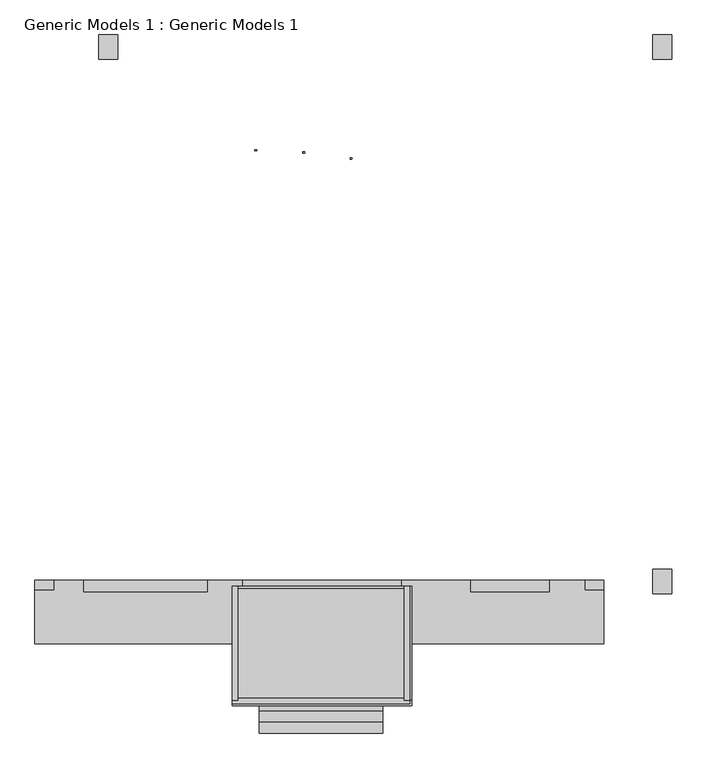
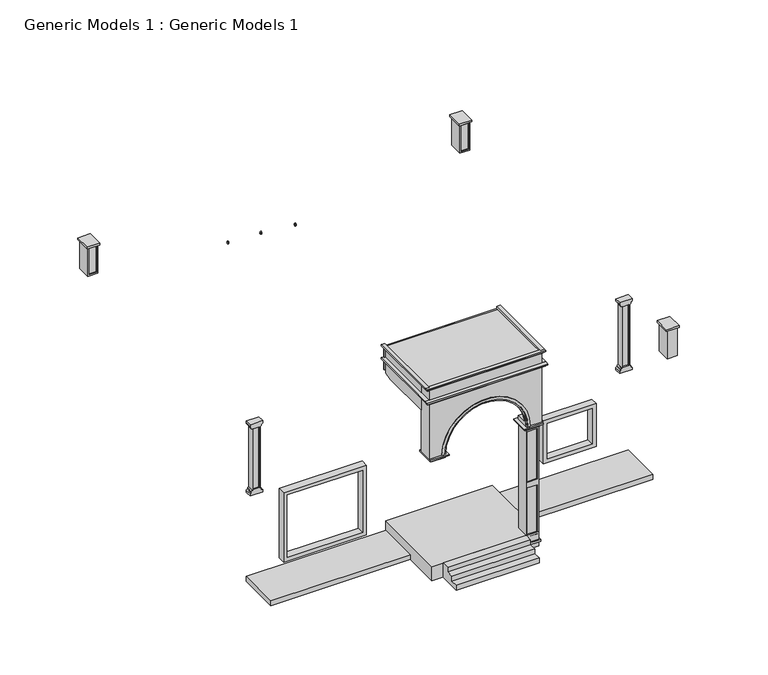
"""IFC4 building model written with IfcOpenShell, lengths in millimetres: proxy geometry, Generic Models 1 : Generic Models 1."""

from ifc_helpers import new_model, si_unit, point, frame, frame_2d, origin, origin_with_axes, place, context, project, spatial, polyline, circle_curve, trimmed, segment, composite_curve, outline, extrude, faceted_brep, source, transform, mapped, element, save
from ifc_brep_helpers import plane_surface, cylinder_surface, revolved_surface, advanced_brep


def generic_models_1_generic_models_1_83f40e1e(model_context):
    return source(origin(), model_context, "Body", "SolidModel", [
        extrude(outline(polyline([(8538.8425759, -5773.6524497), (8538.8425759, -6434.0524497), (8030.8425759, -6434.0524497), (8030.8425759, -5773.6524497), (8538.8425759, -5773.6524497)])), frame((0.0, 0.0, 5029.2), z_axis=(0.0, 0.0, 1.0), x_axis=(1.0, 0.0, 0.0)), (0.0, 0.0, 1.0), 76.2),
        extrude(outline(polyline([(8081.6425759, -6383.2524497), (8081.6425759, -5824.4524497), (8488.0425759, -5824.4524497), (8488.0425759, -6383.2524497), (8081.6425759, -6383.2524497)])), frame((0.0, 0.0, 3810.0), z_axis=(0.0, 0.0, 1.0), x_axis=(1.0, 0.0, 0.0)), (0.0, 0.0, 1.0), 1219.2),
        advanced_brep(
        [(-8670.9249265, -6071.7949916, 6654.8), (-8683.6249265, -6071.7949916, 6654.8), (-8721.7249265, -6071.7949916, 6692.9), (-8721.7249265, -6071.7949916, 6731.0), (-8728.0749265, -6071.7949916, 6731.0), (-8772.5249265, -6071.7949916, 6775.45), (-8772.5249265, -6071.7949916, 6858.0), (-8264.5249265, -6071.7949916, 6858.0), (-8264.5249265, -6071.7949916, 6775.45), (-8308.9749265, -6071.7949916, 6731.0), (-8315.3249265, -6071.7949916, 6731.0), (-8315.3249265, -6071.7949916, 6692.9), (-8353.4249265, -6071.7949916, 6654.8), (-8366.1249265, -6071.7949916, 6654.8), (-8366.1249265, -6071.7949916, 4013.2), (-8353.4249265, -6071.7949916, 4013.2), (-8315.3249265, -6071.7949916, 3975.1), (-8315.3249265, -6071.7949916, 3937.0), (-8308.9749265, -6071.7949916, 3937.0), (-8264.5249265, -6071.7949916, 3892.55), (-8264.5249265, -6071.7949916, 3810.0), (-8772.5249265, -6071.7949916, 3810.0), (-8772.5249265, -6071.7949916, 3892.55), (-8728.0749265, -6071.7949916, 3937.0), (-8721.7249265, -6071.7949916, 3937.0), (-8721.7249265, -6071.7949916, 3975.1), (-8683.6249265, -6071.7949916, 4013.2), (-8670.9249265, -6071.7949916, 4013.2), (-8670.9249265, -6332.4524497, 6654.8), (-8670.9249265, -6332.4524497, 4013.2), (-8683.6249265, -6332.4524497, 4013.2), (-8721.7249265, -6332.4524497, 3975.1), (-8721.7249265, -6332.4524497, 3937.0), (-8728.0749265, -6332.4524497, 3937.0), (-8772.5249265, -6332.4524497, 3892.55), (-8772.5249265, -6332.4524497, 3810.0), (-8264.5249265, -6332.4524497, 3810.0), (-8264.5249265, -6332.4524497, 3892.55), (-8308.9749265, -6332.4524497, 3937.0), (-8315.3249265, -6332.4524497, 3937.0), (-8315.3249265, -6332.4524497, 3975.1), (-8353.4249265, -6332.4524497, 4013.2), (-8366.1249265, -6332.4524497, 4013.2), (-8366.1249265, -6332.4524497, 6654.8), (-8353.4249265, -6332.4524497, 6654.8), (-8315.3249265, -6332.4524497, 6692.9), (-8315.3249265, -6332.4524497, 6731.0), (-8308.9749265, -6332.4524497, 6731.0), (-8264.5249265, -6332.4524497, 6775.45), (-8264.5249265, -6332.4524497, 6858.0), (-8772.5249265, -6332.4524497, 6858.0), (-8772.5249265, -6332.4524497, 6775.45), (-8728.0749265, -6332.4524497, 6731.0), (-8721.7249265, -6332.4524497, 6731.0), (-8721.7249265, -6332.4524497, 6692.9), (-8683.6249265, -6332.4524497, 6654.8), (-8391.5249265, -6332.4524497, 6629.4), (-8391.5249265, -6332.4524497, 4038.6), (-8645.5249265, -6332.4524497, 4038.6), (-8645.5249265, -6332.4524497, 6629.4), (-8391.5249265, -6281.6524497, 6629.4), (-8645.5249265, -6281.6524497, 6629.4), (-8645.5249265, -6281.6524497, 4038.6), (-8391.5249265, -6281.6524497, 4038.6)],
        [
            (0, 1),
            (1, 2, circle_curve(frame((-8683.6249265, -6071.7949916, 6692.9), z_axis=(0.0, 1.0, 0.0), x_axis=(-1.0, 0.0, 0.0)), 38.1)),
            (2, 3),
            (3, 4),
            (4, 5, circle_curve(frame((-8728.0749265, -6071.7949916, 6775.45), z_axis=(0.0, 1.0, 0.0), x_axis=(-1.0, 0.0, 0.0)), 44.45)),
            (5, 6),
            (6, 7),
            (7, 8),
            (8, 9, circle_curve(frame((-8308.9749265, -6071.7949916, 6775.45), z_axis=(0.0, 1.0, 0.0), x_axis=(1.0, 0.0, 0.0)), 44.45)),
            (9, 10),
            (10, 11),
            (11, 12, circle_curve(frame((-8353.4249265, -6071.7949916, 6692.9), z_axis=(0.0, 1.0, 0.0), x_axis=(1.0, 0.0, 0.0)), 38.1)),
            (12, 13),
            (13, 14),
            (14, 15),
            (15, 16, circle_curve(frame((-8353.4249265, -6071.7949916, 3975.1), z_axis=(0.0, 1.0, 0.0), x_axis=(1.0, 0.0, 0.0)), 38.1)),
            (16, 17),
            (17, 18),
            (18, 19, circle_curve(frame((-8308.9749265, -6071.7949916, 3892.55), z_axis=(0.0, 1.0, 0.0), x_axis=(1.0, 0.0, 0.0)), 44.45)),
            (19, 20),
            (20, 21),
            (21, 22),
            (22, 23, circle_curve(frame((-8728.0749265, -6071.7949916, 3892.55), z_axis=(0.0, 1.0, 0.0), x_axis=(-1.0, 0.0, 0.0)), 44.45)),
            (23, 24),
            (24, 25),
            (25, 26, circle_curve(frame((-8683.6249265, -6071.7949916, 3975.1), z_axis=(0.0, 1.0, 0.0), x_axis=(-1.0, 0.0, 0.0)), 38.1)),
            (26, 27),
            (27, 0),
            (28, 29),
            (29, 30),
            (30, 31, circle_curve(frame((-8683.6249265, -6332.4524497, 3975.1), z_axis=(0.0, -1.0, 0.0), x_axis=(-1.0, 0.0, 0.0)), 38.1)),
            (31, 32),
            (32, 33),
            (33, 34, circle_curve(frame((-8728.0749265, -6332.4524497, 3892.55), z_axis=(0.0, -1.0, 0.0), x_axis=(-1.0, 0.0, 0.0)), 44.45)),
            (34, 35),
            (35, 36),
            (36, 37),
            (37, 38, circle_curve(frame((-8308.9749265, -6332.4524497, 3892.55), z_axis=(0.0, -1.0, 0.0), x_axis=(1.0, 0.0, 0.0)), 44.45)),
            (38, 39),
            (39, 40),
            (40, 41, circle_curve(frame((-8353.4249265, -6332.4524497, 3975.1), z_axis=(0.0, -1.0, 0.0), x_axis=(1.0, 0.0, 0.0)), 38.1)),
            (41, 42),
            (42, 43),
            (43, 44),
            (44, 45, circle_curve(frame((-8353.4249265, -6332.4524497, 6692.9), z_axis=(0.0, -1.0, 0.0), x_axis=(1.0, 0.0, 0.0)), 38.1)),
            (45, 46),
            (46, 47),
            (47, 48, circle_curve(frame((-8308.9749265, -6332.4524497, 6775.45), z_axis=(0.0, -1.0, 0.0), x_axis=(1.0, 0.0, 0.0)), 44.45)),
            (48, 49),
            (49, 50),
            (50, 51),
            (51, 52, circle_curve(frame((-8728.0749265, -6332.4524497, 6775.45), z_axis=(0.0, -1.0, 0.0), x_axis=(-1.0, 0.0, 0.0)), 44.45)),
            (52, 53),
            (53, 54),
            (54, 55, circle_curve(frame((-8683.6249265, -6332.4524497, 6692.9), z_axis=(0.0, -1.0, 0.0), x_axis=(-1.0, 0.0, 0.0)), 38.1)),
            (55, 28),
            (56, 57),
            (57, 58),
            (58, 59),
            (59, 56),
            (0, 28),
            (55, 1),
            (54, 2),
            (53, 3),
            (52, 4),
            (51, 5),
            (50, 6),
            (49, 7),
            (48, 8),
            (47, 9),
            (46, 10),
            (45, 11),
            (44, 12),
            (43, 13),
            (42, 14),
            (41, 15),
            (40, 16),
            (39, 17),
            (38, 18),
            (37, 19),
            (36, 20),
            (35, 21),
            (34, 22),
            (33, 23),
            (32, 24),
            (31, 25),
            (30, 26),
            (29, 27),
            (60, 61),
            (61, 62),
            (62, 63),
            (63, 60),
            (63, 57),
            (56, 60),
            (62, 58),
            (61, 59),
        ],
        [
            plane_surface(frame((-8670.9249265, -6071.7949916, 6654.8), z_axis=(0.0, 1.0, 0.0), x_axis=(-1.0, 0.0, 0.0))),
            plane_surface(frame((-8670.9249265, -6332.4524497, 6654.8), z_axis=(0.0, -1.0, 0.0), x_axis=(1.0, 0.0, 0.0))),
            plane_surface(frame((-8670.9249265, -6071.7949916, 6654.8), z_axis=(0.0, 0.0, -1.0), x_axis=(0.0, -1.0, 0.0))),
            cylinder_surface(frame((-8683.6249265, -6332.4524497, 6692.9), z_axis=(0.0, 1.0, 0.0), x_axis=(-1.0, 0.0, 0.0)), 38.1),
            plane_surface(frame((-8721.7249265, -6071.7949916, 6692.9), z_axis=(-1.0, 0.0, 0.0), x_axis=(0.0, -1.0, 0.0))),
            plane_surface(frame((-8721.7249265, -6071.7949916, 6731.0), z_axis=(0.0, 0.0, -1.0), x_axis=(0.0, -1.0, 0.0))),
            cylinder_surface(frame((-8728.0749265, -6332.4524497, 6775.45), z_axis=(0.0, 1.0, 0.0), x_axis=(-1.0, 0.0, 0.0)), 44.45),
            plane_surface(frame((-8772.5249265, -6071.7949916, 6775.45), z_axis=(-1.0, 0.0, 0.0), x_axis=(0.0, -1.0, 0.0))),
            plane_surface(frame((-8772.5249265, -6071.7949916, 6858.0), z_axis=(0.0, 0.0, 1.0), x_axis=(0.0, -1.0, 0.0))),
            plane_surface(frame((-8264.5249265, -6071.7949916, 6858.0), z_axis=(1.0, 0.0, 0.0), x_axis=(0.0, -1.0, 0.0))),
            cylinder_surface(frame((-8308.9749265, -6332.4524497, 6775.45), z_axis=(0.0, 1.0, 0.0), x_axis=(1.0, 0.0, 0.0)), 44.45),
            plane_surface(frame((-8308.9749265, -6071.7949916, 6731.0), z_axis=(0.0, 0.0, -1.0), x_axis=(0.0, -1.0, 0.0))),
            plane_surface(frame((-8315.3249265, -6071.7949916, 6731.0), z_axis=(1.0, 0.0, 0.0), x_axis=(0.0, -1.0, 0.0))),
            cylinder_surface(frame((-8353.4249265, -6332.4524497, 6692.9), z_axis=(0.0, 1.0, 0.0), x_axis=(1.0, 0.0, 0.0)), 38.1),
            plane_surface(frame((-8353.4249265, -6071.7949916, 6654.8), z_axis=(0.0, 0.0, -1.0), x_axis=(0.0, -1.0, 0.0))),
            plane_surface(frame((-8366.1249265, -6071.7949916, 6654.8), z_axis=(1.0, 0.0, 0.0), x_axis=(0.0, -1.0, 0.0))),
            plane_surface(frame((-8366.1249265, -6071.7949916, 4013.2), z_axis=(0.0, 0.0, 1.0), x_axis=(0.0, -1.0, 0.0))),
            cylinder_surface(frame((-8353.4249265, -6332.4524497, 3975.1), z_axis=(0.0, 1.0, 0.0), x_axis=(1.0, 0.0, 0.0)), 38.1),
            plane_surface(frame((-8315.3249265, -6071.7949916, 3975.1), z_axis=(1.0, 0.0, 0.0), x_axis=(0.0, -1.0, 0.0))),
            plane_surface(frame((-8315.3249265, -6071.7949916, 3937.0), z_axis=(0.0, 0.0, 1.0), x_axis=(0.0, -1.0, 0.0))),
            cylinder_surface(frame((-8308.9749265, -6332.4524497, 3892.55), z_axis=(0.0, 1.0, 0.0), x_axis=(1.0, 0.0, 0.0)), 44.45),
            plane_surface(frame((-8264.5249265, -6071.7949916, 3892.55), z_axis=(1.0, 0.0, 0.0), x_axis=(0.0, -1.0, 0.0))),
            plane_surface(frame((-8264.5249265, -6071.7949916, 3810.0), z_axis=(0.0, 0.0, -1.0), x_axis=(0.0, -1.0, 0.0))),
            plane_surface(frame((-8772.5249265, -6071.7949916, 3810.0), z_axis=(-1.0, 0.0, 0.0), x_axis=(0.0, -1.0, 0.0))),
            cylinder_surface(frame((-8728.0749265, -6332.4524497, 3892.55), z_axis=(0.0, 1.0, 0.0), x_axis=(-1.0, 0.0, 0.0)), 44.45),
            plane_surface(frame((-8728.0749265, -6071.7949916, 3937.0), z_axis=(0.0, 0.0, 1.0), x_axis=(0.0, -1.0, 0.0))),
            plane_surface(frame((-8721.7249265, -6071.7949916, 3937.0), z_axis=(-1.0, 0.0, 0.0), x_axis=(0.0, -1.0, 0.0))),
            cylinder_surface(frame((-8683.6249265, -6332.4524497, 3975.1), z_axis=(0.0, 1.0, 0.0), x_axis=(-1.0, 0.0, 0.0)), 38.1),
            plane_surface(frame((-8683.6249265, -6071.7949916, 4013.2), z_axis=(0.0, 0.0, 1.0), x_axis=(0.0, -1.0, 0.0))),
            plane_surface(frame((-8670.9249265, -6071.7949916, 4013.2), z_axis=(-1.0, 0.0, 0.0), x_axis=(0.0, -1.0, 0.0))),
            plane_surface(frame((-8391.5249265, -6281.6524497, 6629.4), z_axis=(0.0, -1.0, 0.0), x_axis=(0.0, 0.0, -1.0))),
            plane_surface(frame((-8391.5249265, -6281.6524497, 6629.4), z_axis=(-1.0, 0.0, 0.0), x_axis=(0.0, -1.0, 0.0))),
            plane_surface(frame((-8391.5249265, -6281.6524497, 4038.6), z_axis=(0.0, 0.0, 1.0), x_axis=(0.0, -1.0, 0.0))),
            plane_surface(frame((-8645.5249265, -6281.6524497, 4038.6), z_axis=(1.0, 0.0, 0.0), x_axis=(0.0, -1.0, 0.0))),
            plane_surface(frame((-8645.5249265, -6281.6524497, 6629.4), z_axis=(0.0, 0.0, -1.0), x_axis=(0.0, -1.0, 0.0))),
        ],
        [
            (0, [[1, 2, 3, 4, 5, 6, 7, 8, 9, 10, 11, 12, 13, 14, 15, 16, 17, 18, 19, 20, 21, 22, 23, 24, 25, 26, 27, 28]]),
            (1, [[29, 30, 31, 32, 33, 34, 35, 36, 37, 38, 39, 40, 41, 42, 43, 44, 45, 46, 47, 48, 49, 50, 51, 52, 53, 54, 55, 56], [57, 58, 59, 60]]),
            (2, [[-1, 61, -56, 62]]),
            (3, [[-2, -62, -55, 63]]),
            (4, [[-3, -63, -54, 64]]),
            (5, [[-4, -64, -53, 65]]),
            (6, [[-5, -65, -52, 66]]),
            (7, [[-6, -66, -51, 67]]),
            (8, [[-7, -67, -50, 68]]),
            (9, [[-8, -68, -49, 69]]),
            (10, [[-9, -69, -48, 70]]),
            (11, [[-10, -70, -47, 71]]),
            (12, [[-11, -71, -46, 72]]),
            (13, [[-12, -72, -45, 73]]),
            (14, [[-13, -73, -44, 74]]),
            (15, [[-14, -74, -43, 75]]),
            (16, [[-15, -75, -42, 76]]),
            (17, [[-16, -76, -41, 77]]),
            (18, [[-17, -77, -40, 78]]),
            (19, [[-18, -78, -39, 79]]),
            (20, [[-19, -79, -38, 80]]),
            (21, [[-20, -80, -37, 81]]),
            (22, [[-21, -81, -36, 82]]),
            (23, [[-22, -82, -35, 83]]),
            (24, [[-23, -83, -34, 84]]),
            (25, [[-24, -84, -33, 85]]),
            (26, [[-25, -85, -32, 86]]),
            (27, [[-26, -86, -31, 87]]),
            (28, [[-27, -87, -30, 88]]),
            (29, [[-28, -88, -29, -61]]),
            (30, [[89, 90, 91, 92]]),
            (31, [[-92, 93, -57, 94]]),
            (32, [[-91, 95, -58, -93]]),
            (33, [[-90, 96, -59, -95]]),
            (34, [[-89, -94, -60, -96]]),
        ],
    ),
        advanced_brep(
        [(6289.6750735, -6071.7949916, 6654.8), (6276.9750735, -6071.7949916, 6654.8), (6238.8750735, -6071.7949916, 6692.9), (6238.8750735, -6071.7949916, 6731.0), (6232.5250735, -6071.7949916, 6731.0), (6188.0750735, -6071.7949916, 6775.45), (6188.0750735, -6071.7949916, 6858.0), (6696.0750735, -6071.7949916, 6858.0), (6696.0750735, -6071.7949916, 6775.45), (6651.6250735, -6071.7949916, 6731.0), (6645.2750735, -6071.7949916, 6731.0), (6645.2750735, -6071.7949916, 6692.9), (6607.1750735, -6071.7949916, 6654.8), (6594.4750735, -6071.7949916, 6654.8), (6594.4750735, -6071.7949916, 4013.2), (6607.1750735, -6071.7949916, 4013.2), (6645.2750735, -6071.7949916, 3975.1), (6645.2750735, -6071.7949916, 3937.0), (6651.6250735, -6071.7949916, 3937.0), (6696.0750735, -6071.7949916, 3892.55), (6696.0750735, -6071.7949916, 3810.0), (6188.0750735, -6071.7949916, 3810.0), (6188.0750735, -6071.7949916, 3892.55), (6232.5250735, -6071.7949916, 3937.0), (6238.8750735, -6071.7949916, 3937.0), (6238.8750735, -6071.7949916, 3975.1), (6276.9750735, -6071.7949916, 4013.2), (6289.6750735, -6071.7949916, 4013.2), (6289.6750735, -6332.4524497, 6654.8), (6289.6750735, -6332.4524497, 4013.2), (6276.9750735, -6332.4524497, 4013.2), (6238.8750735, -6332.4524497, 3975.1), (6238.8750735, -6332.4524497, 3937.0), (6232.5250735, -6332.4524497, 3937.0), (6188.0750735, -6332.4524497, 3892.55), (6188.0750735, -6332.4524497, 3810.0), (6696.0750735, -6332.4524497, 3810.0), (6696.0750735, -6332.4524497, 3892.55), (6651.6250735, -6332.4524497, 3937.0), (6645.2750735, -6332.4524497, 3937.0), (6645.2750735, -6332.4524497, 3975.1), (6607.1750735, -6332.4524497, 4013.2), (6594.4750735, -6332.4524497, 4013.2), (6594.4750735, -6332.4524497, 6654.8), (6607.1750735, -6332.4524497, 6654.8), (6645.2750735, -6332.4524497, 6692.9), (6645.2750735, -6332.4524497, 6731.0), (6651.6250735, -6332.4524497, 6731.0), (6696.0750735, -6332.4524497, 6775.45), (6696.0750735, -6332.4524497, 6858.0), (6188.0750735, -6332.4524497, 6858.0), (6188.0750735, -6332.4524497, 6775.45), (6232.5250735, -6332.4524497, 6731.0), (6238.8750735, -6332.4524497, 6731.0), (6238.8750735, -6332.4524497, 6692.9), (6276.9750735, -6332.4524497, 6654.8), (6569.0750735, -6332.4524497, 6629.4), (6569.0750735, -6332.4524497, 4038.6), (6315.0750735, -6332.4524497, 4038.6), (6315.0750735, -6332.4524497, 6629.4), (6569.0750735, -6281.6524497, 6629.4), (6315.0750735, -6281.6524497, 6629.4), (6315.0750735, -6281.6524497, 4038.6), (6569.0750735, -6281.6524497, 4038.6)],
        [
            (0, 1),
            (1, 2, circle_curve(frame((6276.9750735, -6071.7949916, 6692.9), z_axis=(0.0, 1.0, 0.0), x_axis=(-1.0, 0.0, 0.0)), 38.1)),
            (2, 3),
            (3, 4),
            (4, 5, circle_curve(frame((6232.5250735, -6071.7949916, 6775.45), z_axis=(0.0, 1.0, 0.0), x_axis=(-1.0, 0.0, 0.0)), 44.45)),
            (5, 6),
            (6, 7),
            (7, 8),
            (8, 9, circle_curve(frame((6651.6250735, -6071.7949916, 6775.45), z_axis=(0.0, 1.0, 0.0), x_axis=(1.0, 0.0, 0.0)), 44.45)),
            (9, 10),
            (10, 11),
            (11, 12, circle_curve(frame((6607.1750735, -6071.7949916, 6692.9), z_axis=(0.0, 1.0, 0.0), x_axis=(1.0, 0.0, 0.0)), 38.1)),
            (12, 13),
            (13, 14),
            (14, 15),
            (15, 16, circle_curve(frame((6607.1750735, -6071.7949916, 3975.1), z_axis=(0.0, 1.0, 0.0), x_axis=(1.0, 0.0, 0.0)), 38.1)),
            (16, 17),
            (17, 18),
            (18, 19, circle_curve(frame((6651.6250735, -6071.7949916, 3892.55), z_axis=(0.0, 1.0, 0.0), x_axis=(1.0, 0.0, 0.0)), 44.45)),
            (19, 20),
            (20, 21),
            (21, 22),
            (22, 23, circle_curve(frame((6232.5250735, -6071.7949916, 3892.55), z_axis=(0.0, 1.0, 0.0), x_axis=(-1.0, 0.0, 0.0)), 44.45)),
            (23, 24),
            (24, 25),
            (25, 26, circle_curve(frame((6276.9750735, -6071.7949916, 3975.1), z_axis=(0.0, 1.0, 0.0), x_axis=(-1.0, 0.0, 0.0)), 38.1)),
            (26, 27),
            (27, 0),
            (28, 29),
            (29, 30),
            (30, 31, circle_curve(frame((6276.9750735, -6332.4524497, 3975.1), z_axis=(0.0, -1.0, 0.0), x_axis=(-1.0, 0.0, 0.0)), 38.1)),
            (31, 32),
            (32, 33),
            (33, 34, circle_curve(frame((6232.5250735, -6332.4524497, 3892.55), z_axis=(0.0, -1.0, 0.0), x_axis=(-1.0, 0.0, 0.0)), 44.45)),
            (34, 35),
            (35, 36),
            (36, 37),
            (37, 38, circle_curve(frame((6651.6250735, -6332.4524497, 3892.55), z_axis=(0.0, -1.0, 0.0), x_axis=(1.0, 0.0, 0.0)), 44.45)),
            (38, 39),
            (39, 40),
            (40, 41, circle_curve(frame((6607.1750735, -6332.4524497, 3975.1), z_axis=(0.0, -1.0, 0.0), x_axis=(1.0, 0.0, 0.0)), 38.1)),
            (41, 42),
            (42, 43),
            (43, 44),
            (44, 45, circle_curve(frame((6607.1750735, -6332.4524497, 6692.9), z_axis=(0.0, -1.0, 0.0), x_axis=(1.0, 0.0, 0.0)), 38.1)),
            (45, 46),
            (46, 47),
            (47, 48, circle_curve(frame((6651.6250735, -6332.4524497, 6775.45), z_axis=(0.0, -1.0, 0.0), x_axis=(1.0, 0.0, 0.0)), 44.45)),
            (48, 49),
            (49, 50),
            (50, 51),
            (51, 52, circle_curve(frame((6232.5250735, -6332.4524497, 6775.45), z_axis=(0.0, -1.0, 0.0), x_axis=(-1.0, 0.0, 0.0)), 44.45)),
            (52, 53),
            (53, 54),
            (54, 55, circle_curve(frame((6276.9750735, -6332.4524497, 6692.9), z_axis=(0.0, -1.0, 0.0), x_axis=(-1.0, 0.0, 0.0)), 38.1)),
            (55, 28),
            (56, 57),
            (57, 58),
            (58, 59),
            (59, 56),
            (0, 28),
            (55, 1),
            (54, 2),
            (53, 3),
            (52, 4),
            (51, 5),
            (50, 6),
            (49, 7),
            (48, 8),
            (47, 9),
            (46, 10),
            (45, 11),
            (44, 12),
            (43, 13),
            (42, 14),
            (41, 15),
            (40, 16),
            (39, 17),
            (38, 18),
            (37, 19),
            (36, 20),
            (35, 21),
            (34, 22),
            (33, 23),
            (32, 24),
            (31, 25),
            (30, 26),
            (29, 27),
            (60, 61),
            (61, 62),
            (62, 63),
            (63, 60),
            (63, 57),
            (56, 60),
            (62, 58),
            (61, 59),
        ],
        [
            plane_surface(frame((-8670.9249265, -6071.7949916, 6654.8), z_axis=(0.0, 1.0, 0.0), x_axis=(-1.0, 0.0, 0.0))),
            plane_surface(frame((-8670.9249265, -6332.4524497, 6654.8), z_axis=(0.0, -1.0, 0.0), x_axis=(1.0, 0.0, 0.0))),
            plane_surface(frame((6289.6750735, -6071.7949916, 6654.8), z_axis=(0.0, 0.0, -1.0), x_axis=(0.0, -1.0, 0.0))),
            cylinder_surface(frame((6276.9750735, -5843.1949916, 6692.9), z_axis=(0.0, 1.0, 0.0), x_axis=(-1.0, 0.0, 0.0)), 38.1),
            plane_surface(frame((6238.8750735, -6071.7949916, 6692.9), z_axis=(-1.0, 0.0, 0.0), x_axis=(0.0, -1.0, 0.0))),
            plane_surface(frame((6238.8750735, -6071.7949916, 6731.0), z_axis=(0.0, 0.0, -1.0), x_axis=(0.0, -1.0, 0.0))),
            cylinder_surface(frame((6232.5250735, -5843.1949916, 6775.45), z_axis=(0.0, 1.0, 0.0), x_axis=(-1.0, 0.0, 0.0)), 44.45),
            plane_surface(frame((6188.0750735, -6071.7949916, 6775.45), z_axis=(-1.0, 0.0, 0.0), x_axis=(0.0, -1.0, 0.0))),
            plane_surface(frame((6188.0750735, -6071.7949916, 6858.0), z_axis=(0.0, 0.0, 1.0), x_axis=(0.0, -1.0, 0.0))),
            plane_surface(frame((6696.0750735, -6071.7949916, 6858.0), z_axis=(1.0, 0.0, 0.0), x_axis=(0.0, -1.0, 0.0))),
            cylinder_surface(frame((6651.6250735, -5843.1949916, 6775.45), z_axis=(0.0, 1.0, 0.0), x_axis=(1.0, 0.0, 0.0)), 44.45),
            plane_surface(frame((6651.6250735, -6071.7949916, 6731.0), z_axis=(0.0, 0.0, -1.0), x_axis=(0.0, -1.0, 0.0))),
            plane_surface(frame((6645.2750735, -6071.7949916, 6731.0), z_axis=(1.0, 0.0, 0.0), x_axis=(0.0, -1.0, 0.0))),
            cylinder_surface(frame((6607.1750735, -5843.1949916, 6692.9), z_axis=(0.0, 1.0, 0.0), x_axis=(1.0, 0.0, 0.0)), 38.1),
            plane_surface(frame((6607.1750735, -6071.7949916, 6654.8), z_axis=(0.0, 0.0, -1.0), x_axis=(0.0, -1.0, 0.0))),
            plane_surface(frame((6594.4750735, -6071.7949916, 6654.8), z_axis=(1.0, 0.0, 0.0), x_axis=(0.0, -1.0, 0.0))),
            plane_surface(frame((6594.4750735, -6071.7949916, 4013.2), z_axis=(0.0, 0.0, 1.0), x_axis=(0.0, -1.0, 0.0))),
            cylinder_surface(frame((6607.1750735, -5843.1949916, 3975.1), z_axis=(0.0, 1.0, 0.0), x_axis=(1.0, 0.0, 0.0)), 38.1),
            plane_surface(frame((6645.2750735, -6071.7949916, 3975.1), z_axis=(1.0, 0.0, 0.0), x_axis=(0.0, -1.0, 0.0))),
            plane_surface(frame((6645.2750735, -6071.7949916, 3937.0), z_axis=(0.0, 0.0, 1.0), x_axis=(0.0, -1.0, 0.0))),
            cylinder_surface(frame((6651.6250735, -5843.1949916, 3892.55), z_axis=(0.0, 1.0, 0.0), x_axis=(1.0, 0.0, 0.0)), 44.45),
            plane_surface(frame((6696.0750735, -6071.7949916, 3892.55), z_axis=(1.0, 0.0, 0.0), x_axis=(0.0, -1.0, 0.0))),
            plane_surface(frame((6696.0750735, -6071.7949916, 3810.0), z_axis=(0.0, 0.0, -1.0), x_axis=(0.0, -1.0, 0.0))),
            plane_surface(frame((6188.0750735, -6071.7949916, 3810.0), z_axis=(-1.0, 0.0, 0.0), x_axis=(0.0, -1.0, 0.0))),
            cylinder_surface(frame((6232.5250735, -5843.1949916, 3892.55), z_axis=(0.0, 1.0, 0.0), x_axis=(-1.0, 0.0, 0.0)), 44.45),
            plane_surface(frame((6232.5250735, -6071.7949916, 3937.0), z_axis=(0.0, 0.0, 1.0), x_axis=(0.0, -1.0, 0.0))),
            plane_surface(frame((6238.8750735, -6071.7949916, 3937.0), z_axis=(-1.0, 0.0, 0.0), x_axis=(0.0, -1.0, 0.0))),
            cylinder_surface(frame((6276.9750735, -5843.1949916, 3975.1), z_axis=(0.0, 1.0, 0.0), x_axis=(-1.0, 0.0, 0.0)), 38.1),
            plane_surface(frame((6276.9750735, -6071.7949916, 4013.2), z_axis=(0.0, 0.0, 1.0), x_axis=(0.0, -1.0, 0.0))),
            plane_surface(frame((6289.6750735, -6071.7949916, 4013.2), z_axis=(-1.0, 0.0, 0.0), x_axis=(0.0, -1.0, 0.0))),
            plane_surface(frame((-8391.5249265, -6281.6524497, 6629.4), z_axis=(0.0, -1.0, 0.0), x_axis=(0.0, 0.0, -1.0))),
            plane_surface(frame((6569.0750735, -6281.6524497, 6629.4), z_axis=(-1.0, 0.0, 0.0), x_axis=(0.0, -1.0, 0.0))),
            plane_surface(frame((6569.0750735, -6281.6524497, 4038.6), z_axis=(0.0, 0.0, 1.0), x_axis=(0.0, -1.0, 0.0))),
            plane_surface(frame((6315.0750735, -6281.6524497, 4038.6), z_axis=(1.0, 0.0, 0.0), x_axis=(0.0, -1.0, 0.0))),
            plane_surface(frame((6315.0750735, -6281.6524497, 6629.4), z_axis=(0.0, 0.0, -1.0), x_axis=(0.0, -1.0, 0.0))),
        ],
        [
            (0, [[1, 2, 3, 4, 5, 6, 7, 8, 9, 10, 11, 12, 13, 14, 15, 16, 17, 18, 19, 20, 21, 22, 23, 24, 25, 26, 27, 28]]),
            (1, [[29, 30, 31, 32, 33, 34, 35, 36, 37, 38, 39, 40, 41, 42, 43, 44, 45, 46, 47, 48, 49, 50, 51, 52, 53, 54, 55, 56], [57, 58, 59, 60]]),
            (2, [[-1, 61, -56, 62]]),
            (3, [[-2, -62, -55, 63]]),
            (4, [[-3, -63, -54, 64]]),
            (5, [[-4, -64, -53, 65]]),
            (6, [[-5, -65, -52, 66]]),
            (7, [[-6, -66, -51, 67]]),
            (8, [[-7, -67, -50, 68]]),
            (9, [[-8, -68, -49, 69]]),
            (10, [[-9, -69, -48, 70]]),
            (11, [[-10, -70, -47, 71]]),
            (12, [[-11, -71, -46, 72]]),
            (13, [[-12, -72, -45, 73]]),
            (14, [[-13, -73, -44, 74]]),
            (15, [[-14, -74, -43, 75]]),
            (16, [[-15, -75, -42, 76]]),
            (17, [[-16, -76, -41, 77]]),
            (18, [[-17, -77, -40, 78]]),
            (19, [[-18, -78, -39, 79]]),
            (20, [[-19, -79, -38, 80]]),
            (21, [[-20, -80, -37, 81]]),
            (22, [[-21, -81, -36, 82]]),
            (23, [[-22, -82, -35, 83]]),
            (24, [[-23, -83, -34, 84]]),
            (25, [[-24, -84, -33, 85]]),
            (26, [[-25, -85, -32, 86]]),
            (27, [[-26, -86, -31, 87]]),
            (28, [[-27, -87, -30, 88]]),
            (29, [[-28, -88, -29, -61]]),
            (30, [[89, 90, 91, 92]]),
            (31, [[-92, 93, -57, 94]]),
            (32, [[-91, 95, -58, -93]]),
            (33, [[-90, 96, -59, -95]]),
            (34, [[-89, -94, -60, -96]]),
        ],
    ),
        faceted_brep([(-6980.5574241, 8145.5475503, 5029.2), (-6574.1574241, 8145.5475503, 5029.2), (-6574.1574241, 8704.3475503, 5029.2), (-6980.5574241, 8704.3475503, 5029.2), (-6980.5574241, 8145.5475503, 3810.0), (-6980.5574241, 8704.3475503, 3810.0), (-6574.1574241, 8704.3475503, 3810.0), (-6574.1574241, 8145.5475503, 3810.0), (-6624.9574241, 8145.5475503, 4978.4), (-6624.9574241, 8145.5475503, 3860.8), (-6929.7574241, 8145.5475503, 3860.8), (-6929.7574241, 8145.5475503, 4978.4), (-6624.9574241, 8196.3475503, 4978.4), (-6929.7574241, 8196.3475503, 4978.4), (-6929.7574241, 8196.3475503, 3860.8), (-6624.9574241, 8196.3475503, 3860.8)], [[[0, 1, 2, 3]], [[4, 5, 6, 7]], [[1, 0, 4, 7], [8, 9, 10, 11]], [[2, 1, 7, 6]], [[3, 2, 6, 5]], [[0, 3, 5, 4]], [[12, 13, 14, 15]], [[12, 15, 9, 8]], [[15, 14, 10, 9]], [[14, 13, 11, 10]], [[13, 12, 8, 11]]]),
        faceted_brep([(8081.6425759, 8145.5475503, 5029.2), (8488.0425759, 8145.5475503, 5029.2), (8488.0425759, 8704.3475503, 5029.2), (8081.6425759, 8704.3475503, 5029.2), (8081.6425759, 8145.5475503, 3810.0), (8081.6425759, 8704.3475503, 3810.0), (8488.0425759, 8704.3475503, 3810.0), (8488.0425759, 8145.5475503, 3810.0), (8437.2425759, 8145.5475503, 4978.4), (8437.2425759, 8145.5475503, 3860.8), (8132.4425759, 8145.5475503, 3860.8), (8132.4425759, 8145.5475503, 4978.4), (8437.2425759, 8196.3475503, 4978.4), (8132.4425759, 8196.3475503, 4978.4), (8132.4425759, 8196.3475503, 3860.8), (8437.2425759, 8196.3475503, 3860.8)], [[[0, 1, 2, 3]], [[4, 5, 6, 7]], [[1, 0, 4, 7], [8, 9, 10, 11]], [[2, 1, 7, 6]], [[3, 2, 6, 5]], [[0, 3, 5, 4]], [[12, 13, 14, 15]], [[12, 15, 9, 8]], [[15, 14, 10, 9]], [[14, 13, 11, 10]], [[13, 12, 8, 11]]]),
        extrude(outline(polyline([(-6523.3574241, 8755.1475503), (-6523.3574241, 8094.7475503), (-7031.3574241, 8094.7475503), (-7031.3574241, 8755.1475503), (-6523.3574241, 8755.1475503)])), frame((0.0, 0.0, 5029.2), z_axis=(0.0, 0.0, 1.0), x_axis=(1.0, 0.0, 0.0)), (0.0, 0.0, 1.0), 76.2),
        extrude(outline(polyline([(8538.8425759, 8755.1475503), (8538.8425759, 8094.7475503), (8030.8425759, 8094.7475503), (8030.8425759, 8755.1475503), (8538.8425759, 8755.1475503)])), frame((0.0, 0.0, 5029.2), z_axis=(0.0, 0.0, 1.0), x_axis=(1.0, 0.0, 0.0)), (0.0, 0.0, 1.0), 76.2),
        extrude(outline(polyline([(6696.0750735, -6071.7949916), (6696.0750735, -7793.5697181), (1190.1408344, -7793.5697181), (1190.1408344, -6071.7949916), (6696.0750735, -6071.7949916)])), origin_with_axes(), (0.0, 0.0, 1.0), 203.2),
        extrude(outline(polyline([(-8772.5249265, -7793.5697181), (-8772.5249265, -6071.7949916), (-3127.8591656, -6071.7949916), (-3127.8591656, -7793.5697181), (-8772.5249265, -7793.5697181)])), origin_with_axes(), (0.0, 0.0, 1.0), 203.2),
        extrude(outline(polyline([(-9310.2949916, 609.6), (-9310.2949916, 0.0), (-10224.6949916, 0.0), (-10224.6949916, 203.2), (-9919.8949916, 203.2), (-9919.8949916, 406.4), (-9615.0949916, 406.4), (-9615.0949916, 609.6), (-9310.2949916, 609.6)])), frame((-2670.6591656, 0.0, 0.0), z_axis=(1.0, 0.0, 0.0), x_axis=(0.0, 1.0, 0.0)), (0.0, 0.0, 1.0), 3352.8),
        extrude(outline(polyline([(1190.1408344, -9310.2949916), (-3127.8591656, -9310.2949916), (-3127.8591656, -6071.7949916), (1190.1408344, -6071.7949916), (1190.1408344, -9310.2949916)])), origin_with_axes(), (0.0, 0.0, 1.0), 609.6),
        extrude(outline(polyline([(2895.6, 5210.1750735), (2895.6, 3076.5750735), (1066.8, 3076.5750735), (1066.8, 5210.1750735), (2895.6, 5210.1750735)]), holes=[polyline([(2743.2, 5057.7750735), (1219.2, 5057.7750735), (1219.2, 3228.9750735), (2743.2, 3228.9750735), (2743.2, 5057.7750735)])]), frame((0.0, -6376.5949916, 0.0), z_axis=(0.0, 1.0, 0.0), x_axis=(0.0, 0.0, 1.0)), (0.0, 0.0, 1.0), 304.8),
        extrude(outline(polyline([(3505.2, -4086.2249265), (3505.2, -7439.0249265), (533.4, -7439.0249265), (533.4, -4086.2249265), (3505.2, -4086.2249265)]), holes=[polyline([(3352.8, -4238.6249265), (685.8, -4238.6249265), (685.8, -7286.6249265), (3352.8, -7286.6249265), (3352.8, -4238.6249265)])]), frame((0.0, -6376.5949916, 0.0), z_axis=(0.0, 1.0, 0.0), x_axis=(0.0, 0.0, 1.0)), (0.0, 0.0, 1.0), 304.8),
        extrude(outline(composite_curve([segment(trimmed(circle_curve(frame_2d((0.0, -25.4)), 25.4), [point((24.9370637, -30.2273027))], [point((24.4695943, -18.5883223))], False, "CARTESIAN"), True, "CONTINUOUS"), segment(trimmed(circle_curve(frame_2d((49.4066581, -23.415625)), 25.4), [point((24.4695943, -18.5883223))], [point((24.9370637, -30.2273027))], False, "CARTESIAN"), True, "CONTINUOUS")], self_intersect=False)), frame((-201.9812034, 5377.2602275, 5340.1060554), z_axis=(0.17364242709468777, 0.9848087669759373, 0.0), x_axis=(0.0, 0.0, -1.0)), (0.0, 0.0, 1.0), 38.1),
        extrude(outline(composite_curve([segment(trimmed(circle_curve(frame_2d((0.0, -25.4)), 25.4), [point((24.9370637, -30.2273027))], [point((24.4695943, -18.5883224))], False, "CARTESIAN"), True, "CONTINUOUS"), segment(trimmed(circle_curve(frame_2d((49.4066581, -23.4156251)), 25.4), [point((24.4695943, -18.5883224))], [point((24.9370637, -30.2273027))], False, "CARTESIAN"), True, "CONTINUOUS")], self_intersect=False)), frame((-1493.4736142, 5545.1350666, 5340.1060554), z_axis=(0.08715283421686557, 0.996194952550939, 0.0), x_axis=(0.0, 0.0, -1.0)), (0.0, 0.0, 1.0), 38.1),
        extrude(outline(composite_curve([segment(trimmed(circle_curve(frame_2d((5340.1060554, -2769.2826031)), 25.4), [point((5315.1689917, -2764.4553004))], [point((5315.6364611, -2776.0942807))], False, "CARTESIAN"), True, "CONTINUOUS"), segment(trimmed(circle_curve(frame_2d((5290.6993973, -2771.2669781)), 25.4), [point((5315.6364611, -2776.0942807))], [point((5315.1689917, -2764.4553004))], False, "CARTESIAN"), True, "CONTINUOUS")], self_intersect=False)), frame((0.0, 5599.81391, 0.0), z_axis=(0.0, 1.0, 0.0), x_axis=(0.0, 0.0, 1.0)), (0.0, 0.0, 1.0), 38.1),
        extrude(outline(composite_curve([segment(trimmed(circle_curve(frame_2d((5265.2993973, -956.1591656)), 1689.1), [point((5265.2993973, -2645.2591656))], [point((5265.2993973, 732.9408344))], True, "CARTESIAN"), True, "CONTINUOUS"), segment(polyline([(5265.2993973, 732.9408344), (5265.2993973, 834.5408344)]), True, "CONTINUOUS"), segment(trimmed(circle_curve(frame_2d((5265.2993973, -956.1591656)), 1790.7), [point((5265.2993973, 834.5408344))], [point((5265.2993973, -2746.8591656))], False, "CARTESIAN"), True, "CONTINUOUS"), segment(polyline([(5265.2993973, -2746.8591656), (5265.2993973, -2645.2591656)]), True, "CONTINUOUS")], self_intersect=False)), frame((0.0, -9354.7175142, 0.0), z_axis=(0.0, 1.0, 0.0), x_axis=(0.0, 0.0, 1.0)), (0.0, 0.0, 1.0), 25.4),
        extrude(outline(composite_curve([segment(polyline([(5265.2993973, 682.1408344), (5265.2993973, 732.9408344)]), True, "CONTINUOUS"), segment(trimmed(circle_curve(frame_2d((5265.2993973, -956.1591656)), 1689.1), [point((5265.2993973, 732.9408344))], [point((5265.2993973, -2645.2591656))], False, "CARTESIAN"), True, "CONTINUOUS"), segment(polyline([(5265.2993973, -2645.2591656), (5265.2993973, -2594.4591656)]), True, "CONTINUOUS"), segment(trimmed(circle_curve(frame_2d((5265.2993973, -956.1591656)), 1638.3), [point((5265.2993973, -2594.4591656))], [point((5265.2993973, 682.1408344))], True, "CARTESIAN"), True, "CONTINUOUS")], self_intersect=False)), frame((0.0, -9342.0175142, 0.0), z_axis=(0.0, 1.0, 0.0), x_axis=(0.0, 0.0, 1.0)), (0.0, 0.0, 1.0), 12.7),
        extrude(outline(polyline([(-8776.8949916, 6858.0), (-8776.8949916, 8210.7806613), (-6282.056266, 8210.7806613), (-6282.056266, 7103.8962863), (-7480.6467926, 6858.0), (-8776.8949916, 6858.0)])), frame((1012.3408344, 0.0, 0.0), z_axis=(1.0, 0.0, 0.0), x_axis=(0.0, 1.0, 0.0)), (0.0, 0.0, 1.0), 304.8),
        extrude(outline(polyline([(-8776.8949916, 7046.2940967), (-8776.8949916, 8210.7806613), (-6282.056266, 8210.7806613), (-6282.056266, 7114.9296556), (-6616.5977971, 7046.2940967), (-8776.8949916, 7046.2940967)])), frame((-3254.8591656, 0.0, 0.0), z_axis=(1.0, 0.0, 0.0), x_axis=(0.0, 1.0, 0.0)), (0.0, 0.0, 1.0), 304.8),
        extrude(outline(polyline([(-3305.6591656, -6231.256266), (1317.1408344, -6231.256266), (1317.1408344, -6282.056266), (-3305.6591656, -6282.056266), (-3305.6591656, -6231.256266)])), frame((0.0, 0.0, 7261.4556613), z_axis=(0.0, 0.0, 1.0), x_axis=(1.0, 0.0, 0.0)), (0.0, 0.0, 1.0), 1000.125),
        extrude(outline(polyline([(1271.5651866, -9269.4696223), (-3254.8591656, -9269.4696223), (-3254.8591656, -6282.056266), (1271.5651866, -6282.056266), (1271.5651866, -9269.4696223)])), frame((0.0, 0.0, 8210.7806613), z_axis=(0.0, 0.0, 1.0), x_axis=(1.0, 0.0, 0.0)), (0.0, 0.0, 1.0), 50.8),
        faceted_brep([(-3305.6591656, -6231.256266, 8201.2556613), (-3305.6591656, -6231.256266, 8252.0556613), (-3356.4591656, -6231.256266, 8252.0556613), (-3356.4591656, -6231.256266, 8302.8556613), (-3407.2591656, -6231.256266, 8302.8556613), (-3407.2591656, -6231.256266, 8352.2448495), (-3254.8591656, -6231.256266, 8352.2448495), (-3254.8591656, -6231.256266, 8201.2556613), (-3305.6591656, -9329.3175142, 8201.2556613), (-3254.8591656, -9329.3175142, 8201.2556613), (-3254.8591656, -9329.3175142, 8352.2448495), (-3407.2591656, -9329.3175142, 8352.2448495), (-3407.2591656, -9329.3175142, 8302.8556613), (-3356.4591656, -9329.3175142, 8302.8556613), (-3356.4591656, -9329.3175142, 8252.0556613), (-3305.6591656, -9329.3175142, 8252.0556613), (-3305.6591656, -9277.1137795, 8201.2556613), (-3407.2591656, -9277.1137795, 8302.8556613), (-3356.4591656, -9277.1137795, 8302.8556613), (-3356.4591656, -9277.1137795, 8252.0556613), (-3305.6591656, -9277.1137795, 8252.0556613)], [[[0, 1, 2, 3, 4, 5, 6, 7]], [[8, 9, 10, 11, 12, 13, 14, 15]], [[0, 7, 9, 8, 16]], [[7, 6, 10, 9]], [[6, 5, 11, 10]], [[5, 4, 17, 12, 11]], [[4, 3, 18, 13, 12, 17]], [[3, 2, 19, 14, 13, 18]], [[2, 1, 20, 15, 14, 19]], [[1, 0, 16, 8, 15, 20]]]),
        faceted_brep([(1317.1408344, -6231.256266, 8201.2556613), (1266.3408344, -6231.256266, 8201.2556613), (1266.3408344, -6231.256266, 8352.2448495), (1418.7408344, -6231.256266, 8352.2448495), (1418.7408344, -6231.256266, 8302.8556613), (1367.9408344, -6231.256266, 8302.8556613), (1367.9408344, -6231.256266, 8252.0556613), (1317.1408344, -6231.256266, 8252.0556613), (1317.1408344, -9329.3175142, 8201.2556613), (1317.1408344, -9329.3175142, 8252.0556613), (1367.9408344, -9329.3175142, 8252.0556613), (1367.9408344, -9329.3175142, 8302.8556613), (1418.7408344, -9329.3175142, 8302.8556613), (1418.7408344, -9329.3175142, 8352.2448495), (1266.3408344, -9329.3175142, 8352.2448495), (1266.3408344, -9329.3175142, 8201.2556613), (1317.1408344, -9277.1137795, 8201.2556613), (1418.7408344, -9277.1137795, 8352.2448495), (1418.7408344, -9277.1137795, 8302.8556613), (1367.9408344, -9277.1137795, 8302.8556613), (1367.9408344, -9277.1137795, 8252.0556613), (1317.1408344, -9277.1137795, 8252.0556613)], [[[0, 1, 2, 3, 4, 5, 6, 7]], [[8, 9, 10, 11, 12, 13, 14, 15]], [[1, 0, 16, 8, 15]], [[2, 1, 15, 14]], [[3, 2, 14, 13, 17]], [[4, 3, 17, 13, 12, 18]], [[5, 4, 18, 12, 11, 19]], [[6, 5, 19, 11, 10, 20]], [[7, 6, 20, 10, 9, 21]], [[0, 7, 21, 9, 8, 16]]]),
        faceted_brep([(-3407.2591656, -9429.5137795, 8352.2448495), (-3407.2591656, -9277.1137795, 8352.2448495), (-3407.2591656, -9277.1137795, 8302.8556613), (-3407.2591656, -9429.5137795, 8302.8556613), (1317.1431909, -9277.1137795, 8199.8448495), (1317.1431909, -9327.9137795, 8199.8448495), (-3305.6591656, -9327.9137795, 8199.8448495), (-3305.6591656, -9277.1137795, 8199.8448495), (1418.7408344, -9277.1137795, 8352.2448495), (1418.7408344, -9277.1137795, 8302.8556613), (1367.9408344, -9277.1137795, 8302.8556613), (1367.9408344, -9277.1137795, 8252.0619242), (1317.1431909, -9277.1137795, 8252.0619242), (-3305.6591656, -9277.1137795, 8252.0556613), (-3356.4591656, -9277.1137795, 8252.0556613), (-3356.4591656, -9277.1137795, 8302.8556613), (1418.7408344, -9429.5137795, 8352.2448495), (-3356.4591656, -9429.5137795, 8302.8556613), (-3356.4591656, -9429.5137795, 8301.4448495), (1367.9408344, -9429.5137795, 8301.4448495), (1367.9408344, -9429.5137795, 8302.8556613), (1418.7408344, -9429.5137795, 8302.8556613), (1367.9408344, -9378.7137795, 8301.4448495), (-3356.4591656, -9378.7137795, 8301.4448495), (1367.9408344, -9378.7137795, 8252.0619242), (-3356.4591656, -9378.7137795, 8252.0556613), (-3305.6591656, -9378.7137795, 8252.0556613), (-3305.6591656, -9378.7137795, 8250.6448495), (1317.1431909, -9378.7137795, 8250.6448495), (1317.1431909, -9378.7137795, 8252.0619242), (1317.1431909, -9327.9137795, 8250.6448495), (-3305.6591656, -9327.9137795, 8250.6448495)], [[[0, 1, 2, 3]], [[4, 5, 6, 7]], [[1, 8, 9, 10, 11, 12, 4, 7, 13, 14, 15, 2]], [[1, 0, 16, 8]], [[16, 0, 3, 17, 18, 19, 20, 21]], [[22, 19, 18, 23]], [[24, 22, 23, 25, 26, 27, 28, 29]], [[30, 28, 27, 31]], [[5, 30, 31, 6]], [[10, 20, 19, 22, 24, 11]], [[12, 29, 28, 30, 5, 4]], [[21, 9, 8, 16]], [[29, 12, 11, 24]], [[20, 10, 9, 21]], [[26, 13, 7, 6, 31, 27]], [[13, 26, 25, 14]], [[14, 25, 23, 18, 17, 15]], [[15, 17, 3, 2]]]),
        faceted_brep([(1367.9408344, -9329.3175142, 7645.4), (1367.9408344, -9380.1175142, 7645.4), (-3305.6591656, -9380.1175142, 7645.4), (-3305.6591656, -9329.3175142, 7645.4), (1469.5408344, -9329.3175142, 7797.8), (1469.5408344, -9329.3175142, 7747.0), (1418.7408344, -9329.3175142, 7747.0), (1418.7408344, -9329.3175142, 7696.2), (1367.9408344, -9329.3175142, 7696.2), (-3305.6591656, -9329.3175142, 7696.2), (-3356.4591656, -9329.3175142, 7696.2), (-3356.4591656, -9329.3175142, 7747.0), (-3407.2591656, -9329.3175142, 7747.0), (-3407.2591656, -9329.3175142, 7797.8), (1469.5408344, -9481.7175142, 7797.8), (-3407.2591656, -9481.7175142, 7797.8), (-3407.2591656, -9481.7175142, 7747.0), (1469.5408344, -9481.7175142, 7747.0), (1418.7408344, -9430.9175142, 7747.0), (-3356.4591656, -9430.9175142, 7747.0), (-3356.4591656, -9430.9175142, 7696.2), (1418.7408344, -9430.9175142, 7696.2), (1367.9408344, -9380.1175142, 7696.2), (-3305.6591656, -9380.1175142, 7696.2)], [[[0, 1, 2, 3]], [[4, 5, 6, 7, 8, 0, 3, 9, 10, 11, 12, 13]], [[14, 4, 13, 15]], [[16, 17, 14, 15]], [[18, 6, 5, 17, 16, 12, 11, 19]], [[20, 21, 18, 19]], [[22, 8, 7, 21, 20, 10, 9, 23]], [[1, 22, 23, 2]], [[5, 4, 14, 17]], [[6, 18, 21, 7]], [[8, 22, 1, 0]], [[12, 16, 15, 13]], [[23, 9, 3, 2]], [[19, 11, 10, 20]]]),
        extrude(outline(polyline([(7645.4, -3305.6591656), (7645.4, -3254.8591656), (7797.8, -3254.8591656), (7797.8, -3407.2591656), (7747.0, -3407.2591656), (7747.0, -3356.4591656), (7696.2, -3356.4591656), (7696.2, -3305.6591656), (7645.4, -3305.6591656)])), frame((0.0, -9329.3175142, 0.0), z_axis=(0.0, 1.0, 0.0), x_axis=(0.0, 0.0, 1.0)), (0.0, 0.0, 1.0), 3098.0612483),
        extrude(outline(polyline([(7645.4, 1367.9408344), (7696.2, 1367.9408344), (7696.2, 1418.7408344), (7747.0, 1418.7408344), (7747.0, 1469.5408344), (7797.8, 1469.5408344), (7797.8, 1317.1408344), (7645.4, 1317.1408344), (7645.4, 1367.9408344)])), frame((0.0, -9329.3175142, 0.0), z_axis=(0.0, 1.0, 0.0), x_axis=(0.0, 0.0, 1.0)), (0.0, 0.0, 1.0), 3098.0612483),
        advanced_brep(
        [(-3254.8591656, -8776.8949916, 8210.7806613), (-3254.8591656, -9329.3175142, 8210.7806613), (1317.1408344, -9329.3175142, 8210.7806613), (1317.1408344, -8776.8949916, 8210.7806613), (1012.3408344, -8776.8949916, 8210.7806613), (1012.3408344, -9227.7175142, 8210.7806613), (-2950.0591656, -9227.7175142, 8210.7806613), (-2950.0591656, -8776.8949916, 8210.7806613), (1317.1408344, -8776.8949916, 5265.2993973), (1317.1408344, -9329.3175142, 5265.2993973), (682.1408344, -9329.3175142, 5265.2993973), (682.1408344, -8776.8949916, 5265.2993973), (-3254.8591656, -9329.3175142, 5265.2993973), (-3254.8591656, -8776.8949916, 5265.2993973), (-2594.4591656, -8776.8949916, 5265.2993973), (-2594.4591656, -9329.3175142, 5265.2993973), (-2950.0591656, -8776.8949916, 5437.7614106), (-2585.3564354, -8776.8949916, 5437.7614106), (673.0381042, -8776.8949916, 5437.7614106), (1012.3408344, -8776.8949916, 5437.7614106), (-2585.3564354, -9227.7175142, 5437.7614106), (673.0381042, -9227.7175142, 5437.7614106), (1012.3408344, -9227.7175142, 5437.7614106), (-2950.0591656, -9227.7175142, 5437.7614106)],
        [
            (0, 1),
            (1, 2),
            (2, 3),
            (3, 4),
            (4, 5),
            (5, 6),
            (6, 7),
            (7, 0),
            (8, 9),
            (9, 10),
            (10, 11),
            (11, 8),
            (12, 13),
            (13, 14),
            (14, 15),
            (15, 12),
            (0, 13),
            (12, 1),
            (15, 10, circle_curve(frame((-956.1591656, -9329.3175142, 5265.2993973), z_axis=(0.0, 1.0, 0.0), x_axis=(1.0, 0.0, 0.0)), 1638.3)),
            (9, 2),
            (8, 3),
            (7, 16),
            (16, 17),
            (17, 14, circle_curve(frame((-956.1591656, -8776.8949916, 5265.2993973), z_axis=(0.0, -1.0, 0.0), x_axis=(1.0, 0.0, 0.0)), 1638.3)),
            (11, 18, circle_curve(frame((-956.1591656, -8776.8949916, 5265.2993973), z_axis=(0.0, -1.0, 0.0), x_axis=(1.0, 0.0, 0.0)), 1638.3)),
            (18, 19),
            (19, 4),
            (17, 20),
            (20, 21, circle_curve(frame((-956.1591656, -9227.7175142, 5265.2993973), z_axis=(0.0, 1.0, 0.0), x_axis=(1.0, 0.0, 0.0)), 1638.3)),
            (21, 18),
            (22, 5),
            (19, 22),
            (22, 21),
            (20, 23),
            (23, 6),
            (23, 16),
        ],
        [
            plane_surface(frame((-3254.8591656, -9329.3175142, 8210.7806613), z_axis=(0.0, 0.0, 1.0), x_axis=(0.0, -1.0, 0.0))),
            plane_surface(frame((-3254.8591656, -9329.3175142, 5265.2993973), z_axis=(0.0, 0.0, -1.0), x_axis=(0.0, 1.0, 0.0))),
            plane_surface(frame((-3254.8591656, -8776.8949916, 8210.7806613), z_axis=(-1.0, 0.0, 0.0), x_axis=(0.0, 0.0, -1.0))),
            plane_surface(frame((-3254.8591656, -9329.3175142, 8210.7806613), z_axis=(0.0, -1.0, 0.0), x_axis=(0.0, 0.0, -1.0))),
            plane_surface(frame((1317.1408344, -9329.3175142, 8210.7806613), z_axis=(1.0, 0.0, 0.0), x_axis=(0.0, 0.0, -1.0))),
            plane_surface(frame((1317.1408344, -8776.8949916, 8210.7806613), z_axis=(0.0, 1.0, 0.0), x_axis=(0.0, 0.0, -1.0))),
            revolved_surface(polyline([(682.1408343999999, -8776.8949916, 5265.2993973), (682.1408343999999, -9329.3175142, 5265.2993973)]), (-956.1591656, -9329.3175142, 5265.2993973), (0.0, 1.0, 0.0)),
            plane_surface(frame((1012.3408344, -7480.1229837, 5437.7614106), z_axis=(-1.0, 0.0, 0.0), x_axis=(0.0, 0.0, 1.0))),
            plane_surface(frame((1012.3408344, -9227.7175142, 5437.7614106), z_axis=(0.0, 1.0, 0.0), x_axis=(0.0, 0.0, 1.0))),
            plane_surface(frame((-2950.0591656, -9227.7175142, 5437.7614106), z_axis=(1.0, 0.0, 0.0), x_axis=(0.0, 0.0, 1.0))),
            plane_surface(frame((1012.3408344, -9081.6949916, 5437.7614106), z_axis=(0.0, 0.0, 1.0), x_axis=(0.0, -1.0, 0.0))),
        ],
        [
            (0, [[1, 2, 3, 4, 5, 6, 7, 8]]),
            (1, [[9, 10, 11, 12]]),
            (1, [[13, 14, 15, 16]]),
            (2, [[-1, 17, -13, 18]]),
            (3, [[-2, -18, -16, 19, -10, 20]]),
            (4, [[-3, -20, -9, 21]]),
            (5, [[-17, -8, 22, 23, 24, -14]]),
            (5, [[-21, -12, 25, 26, 27, -4]]),
            (6, [[-11, -19, -15, -24, 28, 29, 30, -25]]),
            (7, [[31, -5, -27, 32]]),
            (8, [[-31, 33, -29, 34, 35, -6]]),
            (9, [[-35, 36, -22, -7]]),
            (10, [[-33, -32, -26, -30]]),
            (10, [[-36, -34, -28, -23]]),
        ],
    ),
        faceted_brep([(555.1408344, -9414.8736727, 5265.2993973), (1317.1408344, -9414.8736727, 5265.2993973), (1317.1408344, -8675.2949916, 5265.2993973), (682.1408344, -8675.2949916, 5265.2993973), (555.1408344, -8675.2949916, 5265.2993973), (555.1408344, -9329.3175142, 5265.2993973), (555.1408344, -9414.8736727, 5214.4993973), (555.1408344, -8675.2949916, 5214.4993973), (1317.1408344, -8675.2949916, 5214.4993973), (1317.1408344, -9414.8736727, 5214.4993973)], [[[0, 1, 2, 3, 4, 5]], [[6, 7, 8, 9]], [[1, 0, 6, 9]], [[2, 1, 9, 8]], [[8, 7, 4, 3, 2]], [[7, 6, 0, 5, 4]]]),
        faceted_brep([(-3254.8591656, -9414.8736727, 5265.2993973), (-2492.8591656, -9414.8736727, 5265.2993973), (-2492.8591656, -9329.3175142, 5265.2993973), (-2492.8591656, -8675.2949916, 5265.2993973), (-2594.4591656, -8675.2949916, 5265.2993973), (-3254.8591656, -8675.2949916, 5265.2993973), (-3254.8591656, -9414.8736727, 5214.4993973), (-3254.8591656, -8675.2949916, 5214.4993973), (-2492.8591656, -8675.2949916, 5214.4993973), (-2492.8591656, -9414.8736727, 5214.4993973)], [[[0, 1, 2, 3, 4, 5]], [[6, 7, 8, 9]], [[1, 0, 6, 9]], [[9, 8, 3, 2, 1]], [[8, 7, 5, 4, 3]], [[0, 5, 7, 6]]]),
        faceted_brep([(1190.1408344, -8802.2949916, 5105.4), (682.1408344, -8802.2949916, 5105.4), (682.1408344, -9310.2949916, 5105.4), (1190.1408344, -9310.2949916, 5105.4), (1190.1408344, -8802.2949916, 279.4), (1190.1408344, -9310.2949916, 279.4), (682.1408344, -9310.2949916, 279.4), (682.1408344, -8802.2949916, 279.4), (1139.3408344, -9310.2949916, 532.3431413), (732.9408344, -9310.2949916, 532.3431413), (732.9408344, -9310.2949916, 2624.1375), (1139.3408344, -9310.2949916, 2624.1375), (1139.3408344, -9310.2949916, 5029.2), (1139.3408344, -9310.2949916, 2870.2), (732.9408344, -9310.2949916, 2870.2), (732.9408344, -9310.2949916, 5029.2), (1139.3408344, -9259.4949916, 532.3431413), (1139.3408344, -9259.4949916, 2624.1375), (732.9408344, -9259.4949916, 2624.1375), (732.9408344, -9259.4949916, 532.3431413), (1139.3408344, -9259.4949916, 5029.2), (732.9408344, -9259.4949916, 5029.2), (732.9408344, -9259.4949916, 2870.2), (1139.3408344, -9259.4949916, 2870.2)], [[[0, 1, 2, 3]], [[4, 5, 6, 7]], [[1, 0, 4, 7]], [[2, 1, 7, 6]], [[3, 2, 6, 5], [8, 9, 10, 11], [12, 13, 14, 15]], [[0, 3, 5, 4]], [[16, 17, 18, 19]], [[20, 21, 22, 23]], [[16, 19, 9, 8]], [[19, 18, 10, 9]], [[18, 17, 11, 10]], [[17, 16, 8, 11]], [[20, 23, 13, 12]], [[23, 22, 14, 13]], [[22, 21, 15, 14]], [[21, 20, 12, 15]]]),
        faceted_brep([(1266.3408344, -8726.0949916, 5214.4993973), (605.9408344, -8726.0949916, 5214.4993973), (605.9408344, -9364.0736727, 5214.4993973), (1266.3408344, -9364.0736727, 5214.4993973), (1215.5408344, -8776.8949916, 5105.4), (1215.5408344, -9313.2736727, 5105.4), (656.7408344, -9313.2736727, 5105.4), (656.7408344, -8776.8949916, 5105.4)], [[[0, 1, 2, 3]], [[4, 5, 6, 7]], [[4, 7, 1, 0]], [[7, 6, 2, 1]], [[6, 5, 3, 2]], [[5, 4, 0, 3]]]),
        extrude(outline(polyline([(631.3408344, -9361.0949916), (631.3408344, -8751.4949916), (1240.9408344, -8751.4949916), (1240.9408344, -9361.0949916), (631.3408344, -9361.0949916)])), frame((0.0, 0.0, 203.2), z_axis=(0.0, 0.0, 1.0), x_axis=(1.0, 0.0, 0.0)), (0.0, 0.0, 1.0), 76.2),
        extrude(outline(polyline([(682.1408344, -9310.2949916), (682.1408344, -8802.2949916), (1190.1408344, -8802.2949916), (1190.1408344, -9310.2949916), (682.1408344, -9310.2949916)])), origin_with_axes(), (0.0, 0.0, 1.0), 203.2),
        faceted_brep([(-2543.6591656, -8726.0949916, 5214.4993973), (-3204.0591656, -8726.0949916, 5214.4993973), (-3204.0591656, -9364.0736727, 5214.4993973), (-2543.6591656, -9364.0736727, 5214.4993973), (-2594.4591656, -8776.8949916, 5105.4), (-2594.4591656, -9313.2736727, 5105.4), (-3153.2591656, -9313.2736727, 5105.4), (-3153.2591656, -8776.8949916, 5105.4)], [[[0, 1, 2, 3]], [[4, 5, 6, 7]], [[4, 7, 1, 0]], [[7, 6, 2, 1]], [[6, 5, 3, 2]], [[5, 4, 0, 3]]]),
    ])


if __name__ == "__main__":
    model = new_model("IFC4")
    model_context = context("Model", 3, world=origin())
    ifc_project = project(units=[si_unit("LENGTHUNIT", "METRE", prefix="MILLI")], contexts=[model_context])
    site = spatial("IfcSite", under=ifc_project)
    building = spatial("IfcBuilding", under=site)
    placement = place(None, origin())
    generic_models_1_generic_models_1_shape = generic_models_1_generic_models_1_83f40e1e(model_context)
    element("IfcBuildingElementProxy", 1, Name="Generic Models 1 : Generic Models 1", ObjectType="Generic Models 1 : Generic Models 1", at=placement, inside=building, context=model_context, shape_type="MappedRepresentation", body=[
        mapped(generic_models_1_generic_models_1_shape, transform((0.0, 0.0, 0.0), x_axis=(1.0, 0.0, 0.0), y_axis=(0.0, 1.0, 0.0), z_axis=(0.0, 0.0, 1.0))),
    ])
    save(model, "model.ifc")

# Revit data of these elements
# Element 1 (IfcBuildingElementProxy, "Generic Models 1 : Generic Models 1")
#   Materials on its faces: "Laminate, Ivory, Matte", "Earth"
# Materials
#   "Laminate, Ivory, Matte": class "Plastic", colour RGB 247 247 239, transparency 0, Description = "Plastic Laminate - Ivory, Matte", Cost = 0
#   "Earth": class "Generic", colour RGB 97 75 62, transparency 0, Description = "Soil", Cost = 0
